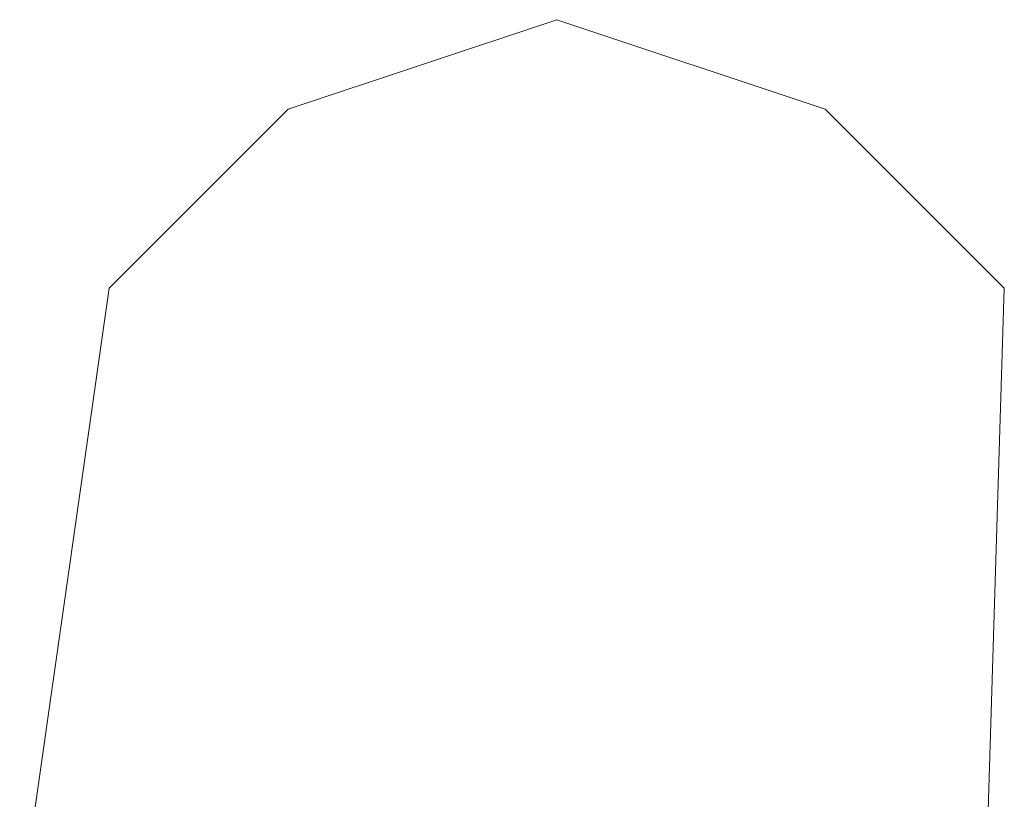
# Model space of a CAD drawing. Units: inches. Extents: x 375 to 1122, y 27 to 1069.
# Tile 16 of 155: x 731.4666 to 732.1437, y 266.6821 to 267.2185. Entities that reach past the tile are written whole.
import ezdxf

# ---------------------------------------------------------------- set-up
doc = ezdxf.new("R2010")
doc.units = ezdxf.units.IN
doc.layers.add('Furniture', color=30, linetype='Continuous', lineweight=18)

# ---------------------------------------------------------------- blocks, each defined once
blk = doc.blocks.new('A$C403C54AD')
for points, invisible_edges in [([(1.978665, 1.176881, -0.053988), (1.978665, 1.167646, -0.053988), (1.981744, 1.164568, -0.053988), (1.981744, 1.17996, -0.053988)], 5), ([(1.978665, 1.176881, -0.055528), (1.978665, 1.167646, -0.055528), (1.981744, 1.164568, -0.055528), (1.981744, 1.17996, -0.055528)], 5), ([(1.981744, 1.17996, -0.053988), (1.981744, 1.17996, -0.055528), (1.978665, 1.176881, -0.055528), (1.978665, 1.176881, -0.053988)], 5), ([(1.981744, 1.164568, -0.053988), (1.981744, 1.17996, -0.053988), (2.030998, 1.178421, -0.053988), (1.992518, 1.163029, -0.053988)], 5), ([(1.981744, 1.164568, -0.055528), (1.981744, 1.17996, -0.055528), (2.030998, 1.178421, -0.055528), (1.992518, 1.163029, -0.055528)], 5), ([(2.030998, 1.178421, -0.055528), (2.030998, 1.178421, -0.053988), (1.981744, 1.17996, -0.053988), (1.981744, 1.17996, -0.055528)], 5), ([(1.977126, 1.172264, -0.053988), (1.977126, 1.172264, -0.053988), (1.978665, 1.176881, -0.053988), (1.978665, 1.167646, -0.053988)], 4), ([(1.977126, 1.172264, -0.055528), (1.977126, 1.172264, -0.055528), (1.978665, 1.176881, -0.055528), (1.978665, 1.167646, -0.055528)], 4), ([(1.978665, 1.176881, -0.055528), (1.978665, 1.176881, -0.053988), (1.977126, 1.172264, -0.053988), (1.977126, 1.172264, -0.055528)], 1), ([(1.977126, 1.172264, -0.053988), (1.977126, 1.172264, -0.055528), (1.978665, 1.167646, -0.055528), (1.978665, 1.167646, -0.053988)], 4), ([(1.978665, 1.167646, -0.055528), (1.978665, 1.167646, -0.053988), (1.981744, 1.164568, -0.053988), (1.981744, 1.164568, -0.055528)], 5), ([(1.981744, 1.164568, -0.053988), (1.981744, 1.164568, -0.055528), (1.992518, 1.163029, -0.055528), (1.992518, 1.163029, -0.053988)], 5)]:
    blk.add_3dface(points, dxfattribs=dict(invisible_edges=invisible_edges))

msp = doc.modelspace()

# ---------------------------------------------------------------- block references
at = {"layer": 'Furniture', "xscale": 39.9918517141215, "yscale": 39.9918517141215, "zscale": 39.9918517141215, "rotation": 270}
msp.add_blockref('A$C403C54AD', (684.95492, 346.28746, 0.02397), dxfattribs=at)

doc.saveas('drawing.dxf')
